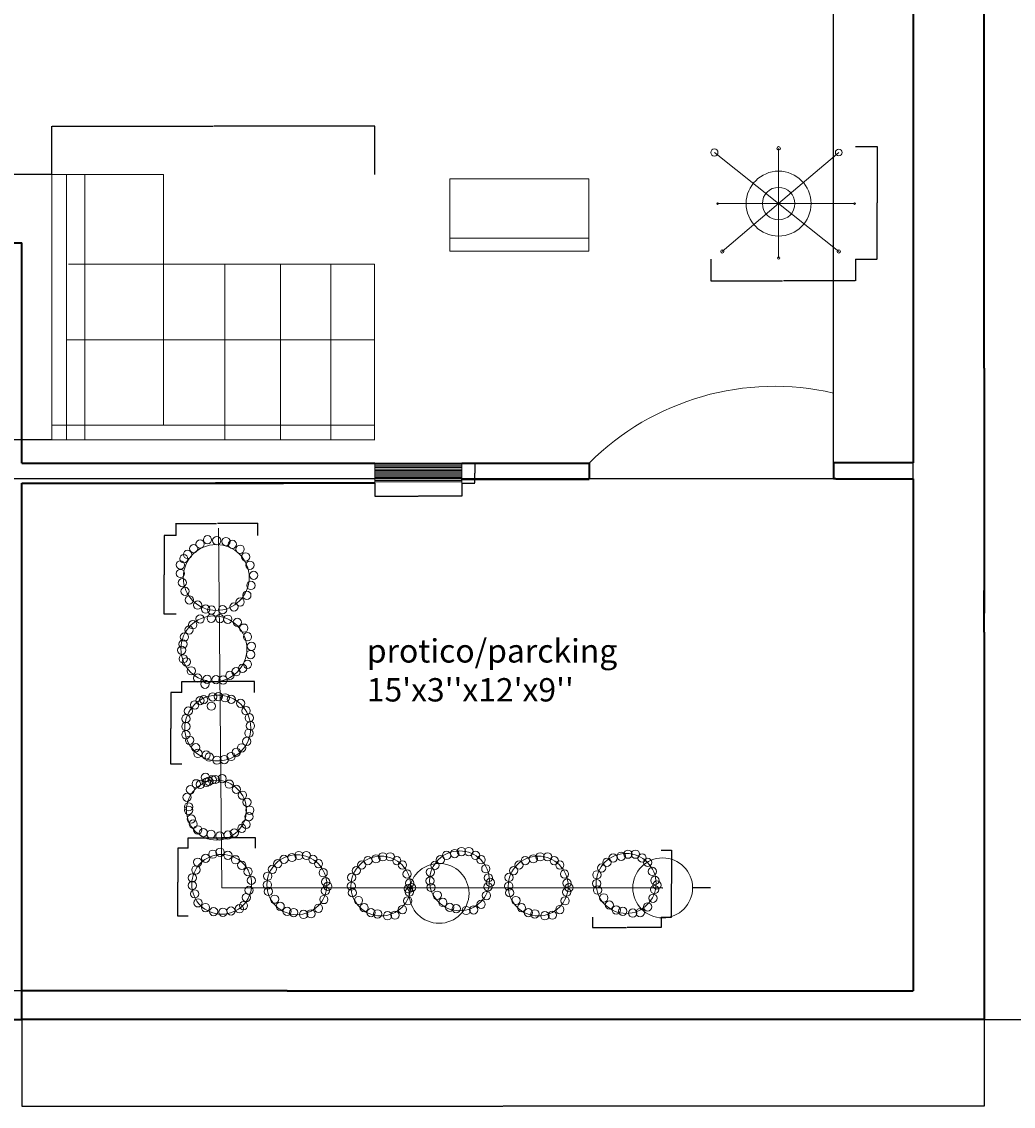
# Model space of a CAD drawing. Units: millimetres. Extents: x 1942 to 12281, y -2698 to 3078.
# Tile 2 of 6: x 4011 to 6981, y -2698 to 552. Entities that reach past the tile are written whole.
import ezdxf

# ---------------------------------------------------------------- set-up
doc = ezdxf.new("R2010")
doc.units = ezdxf.units.MM
for name, color, linetype, lineweight in [('A-ANNO-DIMS', 2, 'Continuous', 18), ('A-AREA-IDEN', 3, 'Continuous', 18), ('A-DOOR', 4, 'Continuous', 18), ('A-FURN', 8, 'Continuous', 18), ('A-GLAZ', 4, 'Continuous', 18), ('A-GLAZ-PATT', 9, 'Continuous', 13), ('A-WALL', 7, 'Continuous', 35), ('E-LITE', 6, 'Continuous', 18), ('L-PLNT', 3, 'Continuous', 13)]:
    doc.layers.add(name, color=color, linetype=linetype, lineweight=lineweight)
doc.styles.get("Standard").update_dxf_attribs({"font": 'arial.ttf'})
doc.dimstyles.get("Standard").update_dxf_attribs({"dimtxt": 0.18, "dimasz": 0.18, "dimexe": 0.18, "dimexo": 0.0625, "dimgap": 0.09, "dimtad": 0, "dimtih": 1, "dimtoh": 1, "dimdec": 4, "dimzin": 0, "dimdsep": 46, "dimtxsty": 'Standard', "dimcen": 0.09, "dimadec": 0, "dimazin": 0, "dimtfac": 1, "dimtdec": 4, "dimtofl": 0, "dimtmove": 0, "dimatfit": 3, "dimfxl": 1, "dimtolj": 1, "dimtzin": 0, "dimarcsym": 0})

# ---------------------------------------------------------------- blocks, each defined once
blk = doc.blocks.new('SOFA-SECTIONAL')
for p, q in [((0, 794.3), (0, 0)), ((0, 794.3), (334.4, 794.3)), ((43.6, 794.3), (43.6, 0)), ((98.1, 794.3), (98.1, 0)), ((334.4, 794.3), (334.4, 43.6)), ((49.7, 525.6), (966.1, 525.6)), ((517.7, 525.6), (517.9, 0)), ((684.1, 525.6), (684.3, 0)), ((834.9, 525.6), (835.1, 0)), ((966.1, 525.6), (966.3, 0)), ((43.6, 299.6), (966.2, 299.6)), ((0, 43.6), (967.4, 43.6)), ((0, 0), (967.4, 0))]:
    blk.add_line(p, q)
blk = doc.blocks.new('SEAT-LIVING')
for p, q in [((0, 38.6), (0, 0)), ((416.9, 0), (416.9, 38.6)), ((0, 0), (416.9, 0))]:
    blk.add_line(p, q)
blk.add_lwpolyline([(0, 217.2), (416.9, 217.2), (416.9, 38.6), (0, 38.6)], close=True)
blk = doc.blocks.new('CHANDELIER-8ARM')
for p, q in [((203.2, 166), (203.2, 331.7)), ((10.7, 319.2), (10.7, 319.2)), ((203.2, 166), (10.7, 319.2)), ((203.2, 166), (383.4, 319.2)), ((203.2, 166), (20.4, 166)), ((203.2, 166), (34.5, 22.7)), ((203.2, 166), (430.7, 166)), ((203.2, 166), (203.2, 3.4)), ((203.2, 166), (383.4, 22.7))]:
    blk.add_line(p, q)
for centre, radius in [((10.7, 319.2), 10.7), ((203.2, 331.7), 5.5), ((383.4, 319.2), 10.2), ((203.2, 166), 97.3), ((203.2, 166), 97.3), ((203.2, 166), 48.7), ((20.4, 166), 2.45), ((430.7, 166), 2.45), ((34.5, 22.7), 4.8), ((203.2, 3.4), 3.36), ((383.4, 22.7), 4.98)]:
    blk.add_circle(centre, radius)
blk = doc.blocks.new('DOOR-ENTRY')
blk.add_line((731.8, 0.7), (731.8, 209.8))
blk.add_arc((555.2, -555.3), 785.2, 77.0012, 134.997)
blk = doc.blocks.new('PLANT-ROUND')
for centre, radius in [((86.1, 183), 12.4), ((106.4, 189), 12.4), ((128.8, 189), 12.4), ((100.7, 101.4), 89.7), ((43.2, 164.4), 12.4), ((61.8, 177.4), 12.4), ((148.6, 177.4), 12.4), ((165.4, 164.4), 12.4), ((13.3, 127.1), 12.4), ((27.3, 147.6), 12.4), ((179.4, 137.3), 12.4), ((12.4, 101), 12.4), ((186.9, 110.3), 12.4), ((193.1, 96.5), 12.4), ((15.2, 81.4), 12.4), ((33.8, 58.1), 12.4), ((181.3, 57.1), 12.4), ((185.9, 83.2), 12.4), ((50.6, 36.6), 12.4), ((71.2, 21.7), 12.4), ((165.4, 31), 12.4), ((90.8, 18), 12.4), ((120.6, 12.4), 12.4), ((143, 14.2), 12.4)]:
    blk.add_circle(centre, radius)
blk = doc.blocks.new('PLANT-ROUND-2')
for centre, radius in [((93.4, 223.1), 12.4), ((121.1, 220.4), 12.4), ((148.7, 217.6), 12.4), ((119.6, 109.8), 98.8), ((52, 196.4), 12.4), ((71.3, 210.2), 12.4), ((168, 209.3), 12.4), ((191, 194.6), 12.4), ((22.5, 166.1), 12.4), ((33.6, 178.9), 12.4), ((207.6, 171.6), 12.4), ((12.4, 147.7), 12.4), ((12.4, 121.9), 12.4), ((220.5, 146.7), 12.4), ((17.9, 94.3), 12.4), ((223.3, 86), 12.4), ((231.6, 116.4), 12.4), ((26.2, 68.5), 12.4), ((211.3, 56.6), 12.4), ((39.1, 42.8), 12.4), ((64, 27.1), 12.4), ((172.6, 21.6), 12.4), ((191, 36.3), 12.4), ((87.9, 15.1), 12.4), ((105.4, 12.4), 12.4), ((138.6, 13.3), 12.4)]:
    blk.add_circle(centre, radius)
blk = doc.blocks.new('PLANT-ROUND-3')
for centre, radius in [((108.8, 118.6), 98.8), ((45.5, 190.7), 12.4), ((67.6, 208.2), 12.4), ((100.8, 210), 12.4), ((126.6, 209.1), 12.4), ((150.5, 207.3), 12.4), ((179.1, 198.1), 12.4), ((20.7, 153.9), 12.4), ((34.5, 175.1), 12.4), ((198.4, 180.6), 12.4), ((209.5, 154.8), 12.4), ((16.1, 132.7), 12.4), ((221.4, 126.3), 12.4), ((12.4, 114.3), 12.4), ((17, 88.6), 12.4), ((218.7, 101.4), 12.4), ((26.2, 79.4), 12.4), ((40.9, 52.7), 12.4), ((194.7, 60), 12.4), ((209.5, 72), 12.4), ((60.1, 30.8), 12.4), ((88.6, 27.1), 12.4), ((115.3, 26.2), 12.4), ((136.5, 25.3), 12.4), ((156.7, 39.1), 12.4), ((175.4, 49.9), 12.4), ((82.2, 12.4), 12.4), ((82.2, 12.4), 12.4), ((82.2, 12.4), 12.4)]:
    blk.add_circle(centre, radius)
blk = doc.blocks.new('PLANT-ROUND-4')
for centre, radius in [((108, 108.9), 98.8), ((54.7, 190.9), 12.4), ((65.8, 193.7), 12.4), ((92.5, 202), 12.4), ((110, 202.9), 12.4), ((130.3, 199.2), 12.4), ((148.7, 194.6), 12.4), ((176.3, 182.6), 12.4), ((19.8, 159.6), 12.4), ((39.1, 178), 12.4), ((88.8, 174.3), 12.4), ((88.8, 174.3), 12.4), ((88.8, 174.3), 12.4), ((88.8, 174.3), 12.4), ((192.9, 160.5), 12.4), ((12.4, 136.6), 12.4), ((202.1, 139.4), 12.4), ((12.4, 113.6), 12.4), ((12.4, 88.8), 12.4), ((201.2, 93.4), 12.4), ((205.8, 115.5), 12.4), ((23.4, 72.2), 12.4), ((194.7, 68.5), 12.4), ((41.9, 50.1), 12.4), ((48.3, 32.6), 12.4), ((73.2, 28), 12.4), ((82.4, 21.6), 12.4), ((147.8, 23.4), 12.4), ((163.4, 36.3), 12.4), ((179.1, 49.2), 12.4), ((105.4, 12.4), 12.4), ((127.5, 14.2), 12.4)]:
    blk.add_circle(centre, radius)
blk = doc.blocks.new('PLANT-ROUND-5')
for centre, radius in [((67.6, 188.1), 12.4), ((117.6, 184.4), 12.4), ((22.5, 151.3), 12.4), ((100.5, 89.8), 89.7), ((40, 168.8), 12.4), ((52, 167), 12.4), ((70.4, 173.4), 12.4), ((77.8, 176.2), 12.4), ((87.9, 180.8), 12.4), ((97.1, 181.7), 12.4), ((138.8, 167.8), 12.4), ((159.9, 152.2), 12.4), ((12.4, 128.3), 12.4), ((178.4, 134.7), 12.4), ((17, 99.8), 12.4), ((17, 89.7), 12.4), ((192.2, 113.5), 12.4), ((200.5, 89.6), 12.4), ((25, 63.2), 12.4), ((25, 63.2), 12.4), ((25, 63.2), 12.4), ((25, 63.2), 12.4), ((25, 63.2), 12.4), ((25, 63.2), 12.4), ((197.7, 70.3), 12.4), ((30.8, 48.3), 12.4), ((44.6, 30.8), 12.4), ((61.2, 22.5), 12.4), ((154.2, 21.6), 12.4), ((176.5, 35.3), 12.4), ((189.4, 47.2), 12.4), ((84.2, 17.9), 12.4), ((110.9, 12.4), 12.4), ((134.9, 15.1), 12.4)]:
    blk.add_circle(centre, radius)
blk = doc.blocks.new('PLANT-ROUND-6')
for centre, radius in [((74, 186.3), 12.4), ((95.8, 192.1), 12.4), ((119.1, 182.8), 12.4), ((100.5, 95.9), 89.7), ((28.8, 162.1), 12.4), ((52.4, 174), 12.4), ((141.9, 169.4), 12.4), ((160.8, 153), 12.4), ((23.3, 139.1), 12.4), ((179.6, 133.8), 12.4), ((12.4, 115.2), 12.4), ((12.4, 92.5), 12.4), ((189.2, 107.7), 12.4), ((19.4, 67.4), 12.4), ((174.3, 56.2), 12.4), ((182.2, 78), 12.4), ((29.6, 40.4), 12.4), ((52, 26.4), 12.4), ((153.8, 22.6), 12.4), ((165.9, 32), 12.4), ((76.3, 14.2), 12.4), ((104.3, 12.4), 12.4), ((128.6, 16.1), 12.4)]:
    blk.add_circle(centre, radius)
blk = doc.blocks.new('WIN-LIVING')
for p, q in [((0, 59.6), (0, 0)), ((0, 59.6), (260.2, 59.6)), ((260.2, 0), (260.2, 59.6))]:
    blk.add_line(p, q)
blk = doc.blocks.new('*D28')
at = {"layer": 'A-ANNO-DIMS', "color": 0, "lineweight": -2, "transparency": 16777216}
for p, q in [((4101.4, 94.2), (4101.4, 239.4)), ((4101.6, 239.3), (4583.8, 239.3)), ((5068.6, 239.3), (4586.5, 239.3)), ((5068.8, 94.2), (5068.8, 239.4))]:
    blk.add_line(p, q, dxfattribs=at)
at = {"layer": 'A-ANNO-DIMS', "color": 0, "transparency": 16777216}
for points in [[(4101.6, 239.3), (4101.6, 239.2), (4101.4, 239.3)], [(5068.6, 239.3), (5068.6, 239.2), (5068.8, 239.3)]]:
    blk.add_solid(points, dxfattribs=at)
at = {"layer": 'Defpoints', "color": 0, "transparency": 16777216}
for p in [(5068.8, 239.3), (4101.4, 94.1), (5068.8, 94.1)]:
    blk.add_point(p, dxfattribs=at)
at = {"layer": 'A-ANNO-DIMS', "color": 0, "transparency": 16777216, "insert": (4585.1, 239.3), "char_height": 0.18, "attachment_point": 5}
blk.add_mtext('\\A1;SECTIONAL 967 TYP.', dxfattribs=at)
blk = doc.blocks.new('*D29')
at = {"layer": 'A-ANNO-DIMS', "color": 0, "lineweight": -2, "transparency": 16777216}
for p, q in [((4101.3, 94.1), (3956.1, 94.1)), ((3956.3, 94), (3956.3, -302.8)), ((3956.3, -700), (3956.3, -303.2)), ((4101.3, -700.2), (3956.1, -700.2))]:
    blk.add_line(p, q, dxfattribs=at)
at = {"layer": 'A-ANNO-DIMS', "color": 0, "transparency": 16777216}
for points in [[(3956.3, 94), (3956.3, 94), (3956.3, 94.1)], [(3956.3, -700), (3956.3, -700), (3956.3, -700.2)]]:
    blk.add_solid(points, dxfattribs=at)
at = {"layer": 'Defpoints', "color": 0, "transparency": 16777216}
for p in [(3956.3, 94.1), (4101.4, 94.1), (4101.4, -700.2)]:
    blk.add_point(p, dxfattribs=at)
at = {"layer": 'A-ANNO-DIMS', "color": 0, "transparency": 16777216, "insert": (3956.3, -303), "char_height": 0.18, "attachment_point": 5}
blk.add_mtext('\\A1;794 TYP.', dxfattribs=at)
blk = doc.blocks.new('*D32')
at = {"layer": 'A-ANNO-DIMS', "color": 0, "lineweight": -2, "transparency": 16777216}
for p, q in [((6075.1, -158.9), (6075.1, -224)), ((6508.2, -158.9), (6508.2, -224)), ((6075.2, -223.8), (6290.2, -223.8)), ((6508, -223.8), (6293.1, -223.8))]:
    blk.add_line(p, q, dxfattribs=at)
at = {"layer": 'A-ANNO-DIMS', "color": 0, "transparency": 16777216}
for points in [[(6075.2, -223.8), (6075.2, -223.9), (6075.1, -223.8)], [(6508, -223.8), (6508, -223.9), (6508.2, -223.8)]]:
    blk.add_solid(points, dxfattribs=at)
at = {"layer": 'Defpoints', "color": 0, "transparency": 16777216}
for p in [(6075.1, -158.9), (6508.2, -158.9), (6508.2, -223.8)]:
    blk.add_point(p, dxfattribs=at)
at = {"layer": 'A-ANNO-DIMS', "color": 0, "transparency": 16777216, "insert": (6291.6, -223.8), "char_height": 0.18, "attachment_point": 5}
blk.add_mtext('\\A1;CHANDELIER 433 TYP.', dxfattribs=at)
blk = doc.blocks.new('*D33')
at = {"layer": 'A-ANNO-DIMS', "color": 0, "lineweight": -2, "transparency": 16777216}
for p, q in [((6508.3, 178.4), (6573.3, 178.4)), ((6573.2, 178.2), (6573.2, 9.9)), ((6573.2, -158.7), (6573.2, 9.6)), ((6508.3, -158.9), (6573.3, -158.9))]:
    blk.add_line(p, q, dxfattribs=at)
at = {"layer": 'A-ANNO-DIMS', "color": 0, "transparency": 16777216}
for points in [[(6573.1, 178.2), (6573.2, 178.2), (6573.2, 178.4)], [(6573.1, -158.7), (6573.2, -158.7), (6573.2, -158.9)]]:
    blk.add_solid(points, dxfattribs=at)
at = {"layer": 'Defpoints', "color": 0, "transparency": 16777216}
for p in [(6508.2, 178.4), (6573.2, 178.4), (6508.2, -158.9)]:
    blk.add_point(p, dxfattribs=at)
at = {"layer": 'A-ANNO-DIMS', "color": 0, "transparency": 16777216, "insert": (6573.2, 9.8), "char_height": 0.18, "attachment_point": 5}
blk.add_mtext('\\A1;337 TYP.', dxfattribs=at)
blk = doc.blocks.new('*D48')
at = {"layer": 'A-ANNO-DIMS', "color": 0, "lineweight": -2, "transparency": 16777216}
for p, q in [((5720.6, -2131.3), (5720.6, -2162.2)), ((5926.1, -2131.3), (5926.1, -2162.2)), ((5720.8, -2162), (5822.2, -2162)), ((5925.9, -2162), (5824.5, -2162))]:
    blk.add_line(p, q, dxfattribs=at)
at = {"layer": 'A-ANNO-DIMS', "color": 0, "transparency": 16777216}
for points in [[(5720.8, -2162), (5720.8, -2162.1), (5720.6, -2162)], [(5925.9, -2162), (5925.9, -2162.1), (5926.1, -2162)]]:
    blk.add_solid(points, dxfattribs=at)
at = {"layer": 'Defpoints', "color": 0, "transparency": 16777216}
for p in [(5720.6, -2131.2), (5926.1, -2131.2), (5926.1, -2162)]:
    blk.add_point(p, dxfattribs=at)
at = {"layer": 'A-ANNO-DIMS', "color": 0, "transparency": 16777216, "insert": (5823.3, -2162), "char_height": 0.18, "attachment_point": 5}
blk.add_mtext('\\A1;PLANT A 205 TYP.', dxfattribs=at)
blk = doc.blocks.new('*D49')
at = {"layer": 'A-ANNO-DIMS', "color": 0, "lineweight": -2, "transparency": 16777216}
for p, q in [((5926.1, -1929.9), (5957.1, -1929.9)), ((5956.9, -1930.1), (5956.9, -2030.4)), ((5956.9, -2131), (5956.9, -2030.7)), ((5926.1, -2131.2), (5957.1, -2131.2))]:
    blk.add_line(p, q, dxfattribs=at)
at = {"layer": 'A-ANNO-DIMS', "color": 0, "transparency": 16777216}
for points in [[(5956.9, -1930.1), (5956.9, -1930.1), (5956.9, -1929.9)], [(5956.9, -2131), (5956.9, -2131), (5956.9, -2131.2)]]:
    blk.add_solid(points, dxfattribs=at)
at = {"layer": 'Defpoints', "color": 0, "transparency": 16777216}
for p in [(5926.1, -1929.9), (5956.9, -1929.9), (5926.1, -2131.2)]:
    blk.add_point(p, dxfattribs=at)
at = {"layer": 'A-ANNO-DIMS', "color": 0, "transparency": 16777216, "insert": (5956.9, -2030.5), "char_height": 0.18, "attachment_point": 5}
blk.add_mtext('\\A1;201 TYP.', dxfattribs=at)
blk = doc.blocks.new('*D50')
at = {"layer": 'A-ANNO-DIMS', "color": 0, "lineweight": -2, "transparency": 16777216}
for p, q in [((4473.9, -987.4), (4473.9, -950.7)), ((4474.1, -950.9), (4594.7, -950.9)), ((4717.7, -950.9), (4597, -950.9)), ((4717.9, -987.4), (4717.9, -950.7))]:
    blk.add_line(p, q, dxfattribs=at)
at = {"layer": 'A-ANNO-DIMS', "color": 0, "transparency": 16777216}
for points in [[(4474.1, -950.9), (4474.1, -950.9), (4473.9, -950.9)], [(4717.7, -950.9), (4717.7, -950.9), (4717.9, -950.9)]]:
    blk.add_solid(points, dxfattribs=at)
at = {"layer": 'Defpoints', "color": 0, "transparency": 16777216}
for p in [(4717.9, -950.9), (4473.9, -987.5), (4717.9, -987.5)]:
    blk.add_point(p, dxfattribs=at)
at = {"layer": 'A-ANNO-DIMS', "color": 0, "transparency": 16777216, "insert": (4595.9, -950.9), "char_height": 0.18, "attachment_point": 5}
blk.add_mtext('\\A1;PLANT B 244 TYP.', dxfattribs=at)
blk = doc.blocks.new('*D51')
at = {"layer": 'A-ANNO-DIMS', "color": 0, "lineweight": -2, "transparency": 16777216}
for p, q in [((4473.9, -987.5), (4437.1, -987.5)), ((4437.3, -987.7), (4437.3, -1105.1)), ((4437.3, -1222.8), (4437.3, -1105.4)), ((4473.9, -1223), (4437.1, -1223))]:
    blk.add_line(p, q, dxfattribs=at)
at = {"layer": 'A-ANNO-DIMS', "color": 0, "transparency": 16777216}
for points in [[(4437.3, -987.7), (4437.4, -987.7), (4437.3, -987.5)], [(4437.3, -1222.8), (4437.4, -1222.8), (4437.3, -1223)]]:
    blk.add_solid(points, dxfattribs=at)
at = {"layer": 'Defpoints', "color": 0, "transparency": 16777216}
for p in [(4437.3, -987.5), (4473.9, -987.5), (4473.9, -1223)]:
    blk.add_point(p, dxfattribs=at)
at = {"layer": 'A-ANNO-DIMS', "color": 0, "transparency": 16777216, "insert": (4437.3, -1105.2), "char_height": 0.18, "attachment_point": 5}
blk.add_mtext('\\A1;236 TYP.', dxfattribs=at)
blk = doc.blocks.new('*D54')
at = {"layer": 'A-ANNO-DIMS', "color": 0, "lineweight": -2, "transparency": 16777216}
for p, q in [((4490.2, -1457.6), (4490.2, -1424.8)), ((4490.3, -1424.9), (4598.1, -1424.9)), ((4708.1, -1424.9), (4600.4, -1424.9)), ((4708.3, -1457.6), (4708.3, -1424.8))]:
    blk.add_line(p, q, dxfattribs=at)
at = {"layer": 'A-ANNO-DIMS', "color": 0, "transparency": 16777216}
for points in [[(4490.3, -1424.9), (4490.3, -1425), (4490.2, -1424.9)], [(4708.1, -1424.9), (4708.1, -1425), (4708.3, -1424.9)]]:
    blk.add_solid(points, dxfattribs=at)
at = {"layer": 'Defpoints', "color": 0, "transparency": 16777216}
for p in [(4708.3, -1424.9), (4490.2, -1457.7), (4708.3, -1457.7)]:
    blk.add_point(p, dxfattribs=at)
at = {"layer": 'A-ANNO-DIMS', "color": 0, "transparency": 16777216, "insert": (4599.2, -1424.9), "char_height": 0.18, "attachment_point": 5}
blk.add_mtext('\\A1;PLANT D 218 TYP.', dxfattribs=at)
blk = doc.blocks.new('*D55')
at = {"layer": 'A-ANNO-DIMS', "color": 0, "lineweight": -2, "transparency": 16777216}
for p, q in [((4490.1, -1457.7), (4457.3, -1457.7)), ((4457.4, -1457.9), (4457.4, -1565.1)), ((4457.4, -1672.8), (4457.4, -1565.5)), ((4490.1, -1672.9), (4457.3, -1672.9))]:
    blk.add_line(p, q, dxfattribs=at)
at = {"layer": 'A-ANNO-DIMS', "color": 0, "transparency": 16777216}
for points in [[(4457.4, -1457.9), (4457.5, -1457.9), (4457.4, -1457.7)], [(4457.4, -1672.8), (4457.5, -1672.8), (4457.4, -1672.9)]]:
    blk.add_solid(points, dxfattribs=at)
at = {"layer": 'Defpoints', "color": 0, "transparency": 16777216}
for p in [(4457.4, -1457.7), (4490.2, -1457.7), (4490.2, -1672.9)]:
    blk.add_point(p, dxfattribs=at)
at = {"layer": 'A-ANNO-DIMS', "color": 0, "transparency": 16777216, "insert": (4457.4, -1565.3), "char_height": 0.18, "attachment_point": 5}
blk.add_mtext('\\A1;215 TYP.', dxfattribs=at)
blk = doc.blocks.new('*D58')
at = {"layer": 'A-ANNO-DIMS', "color": 0, "lineweight": -2, "transparency": 16777216}
for p, q in [((4509.2, -1923.9), (4478.4, -1923.9)), ((4478.6, -1924.1), (4478.6, -2026)), ((4478.6, -2128.3), (4478.6, -2026.4)), ((4509.2, -2128.4), (4478.4, -2128.4))]:
    blk.add_line(p, q, dxfattribs=at)
at = {"layer": 'A-ANNO-DIMS', "color": 0, "transparency": 16777216}
for points in [[(4478.6, -1924.1), (4478.6, -1924.1), (4478.6, -1923.9)], [(4478.6, -2128.3), (4478.6, -2128.3), (4478.6, -2128.4)]]:
    blk.add_solid(points, dxfattribs=at)
at = {"layer": 'Defpoints', "color": 0, "transparency": 16777216}
for p in [(4478.6, -1923.9), (4509.3, -1923.9), (4509.3, -2128.4)]:
    blk.add_point(p, dxfattribs=at)
at = {"layer": 'A-ANNO-DIMS', "color": 0, "transparency": 16777216, "insert": (4478.6, -2026.2), "char_height": 0.18, "attachment_point": 5}
blk.add_mtext('\\A1;PLANT F 204 TYP.', dxfattribs=at)
blk = doc.blocks.new('*D59')
at = {"layer": 'A-ANNO-DIMS', "color": 0, "lineweight": -2, "transparency": 16777216}
for p, q in [((4509.3, -1923.9), (4509.3, -1893.1)), ((4509.4, -1893.3), (4609.5, -1893.3)), ((4710.7, -1893.3), (4610.7, -1893.3)), ((4710.8, -1923.9), (4710.8, -1893.1))]:
    blk.add_line(p, q, dxfattribs=at)
at = {"layer": 'A-ANNO-DIMS', "color": 0, "transparency": 16777216}
for points in [[(4509.4, -1893.2), (4509.4, -1893.3), (4509.3, -1893.3)], [(4710.7, -1893.2), (4710.7, -1893.3), (4710.8, -1893.3)]]:
    blk.add_solid(points, dxfattribs=at)
at = {"layer": 'Defpoints', "color": 0, "transparency": 16777216}
for p in [(4710.8, -1893.3), (4509.3, -1923.9), (4710.8, -1923.9)]:
    blk.add_point(p, dxfattribs=at)
at = {"layer": 'A-ANNO-DIMS', "color": 0, "transparency": 16777216, "insert": (4610.1, -1893.3), "char_height": 0.18, "attachment_point": 5}
blk.add_mtext('\\A1;202 TYP.', dxfattribs=at)
blk = doc.blocks.new('*D68')
at = {"layer": 'A-ANNO-DIMS', "color": 0, "lineweight": -2, "transparency": 16777216}
for p, q in [((5068.8, -830.1), (5068.8, -869.2)), ((5329.1, -830.1), (5329.1, -869.2)), ((5069, -869.1), (5198.1, -869.1)), ((5328.9, -869.1), (5199.8, -869.1))]:
    blk.add_line(p, q, dxfattribs=at)
at = {"layer": 'A-ANNO-DIMS', "color": 0, "transparency": 16777216}
for points in [[(5069, -869), (5069, -869.1), (5068.8, -869.1)], [(5328.9, -869), (5328.9, -869.1), (5329.1, -869.1)]]:
    blk.add_solid(points, dxfattribs=at)
at = {"layer": 'Defpoints', "color": 0, "transparency": 16777216}
for p in [(5068.8, -830), (5329.1, -830), (5329.1, -869.1)]:
    blk.add_point(p, dxfattribs=at)
at = {"layer": 'A-ANNO-DIMS', "color": 0, "transparency": 16777216, "insert": (5199, -869.1), "char_height": 0.18, "attachment_point": 5}
blk.add_mtext('\\A1;W5 260 TYP.', dxfattribs=at)
blk = doc.blocks.new('*D69')
at = {"layer": 'A-ANNO-DIMS', "color": 0, "lineweight": -2, "transparency": 16777216}
for p, q in [((5329.1, -770.4), (5368.3, -770.4)), ((5368.1, -770.6), (5368.1, -800)), ((5368.1, -829.8), (5368.1, -800.4)), ((5329.1, -830), (5368.3, -830))]:
    blk.add_line(p, q, dxfattribs=at)
at = {"layer": 'A-ANNO-DIMS', "color": 0, "transparency": 16777216}
for points in [[(5368.1, -770.6), (5368.1, -770.6), (5368.1, -770.4)], [(5368.1, -829.8), (5368.1, -829.8), (5368.1, -830)]]:
    blk.add_solid(points, dxfattribs=at)
at = {"layer": 'Defpoints', "color": 0, "transparency": 16777216}
for p in [(5329.1, -770.4), (5368.1, -770.4), (5329.1, -830)]:
    blk.add_point(p, dxfattribs=at)
at = {"layer": 'A-ANNO-DIMS', "color": 0, "transparency": 16777216, "insert": (5368.1, -800.2), "char_height": 0.18, "attachment_point": 5}
blk.add_mtext('\\A1;60 TYP.', dxfattribs=at)
blk = doc.blocks.new('*D71')
at = {"layer": 'A-ANNO-DIMS', "color": 0, "lineweight": -2, "transparency": 16777216}
for p, q in [((6894.2, 2765.9), (7154.5, 2765.9)), ((7154.3, 2765.7), (7154.3, 164.5)), ((7154.3, -2437.1), (7154.3, 164.1)), ((6894.2, -2437.2), (7154.5, -2437.2))]:
    blk.add_line(p, q, dxfattribs=at)
at = {"layer": 'A-ANNO-DIMS', "color": 0, "transparency": 16777216}
for points in [[(7154.3, 2765.7), (7154.4, 2765.7), (7154.3, 2765.9)], [(7154.3, -2437.1), (7154.4, -2437.1), (7154.3, -2437.2)]]:
    blk.add_solid(points, dxfattribs=at)
at = {"layer": 'Defpoints', "color": 0, "transparency": 16777216}
for p in [(6894.1, 2765.9), (7154.3, 2765.9), (6894.1, -2437.2)]:
    blk.add_point(p, dxfattribs=at)
at = {"layer": 'A-ANNO-DIMS', "color": 0, "transparency": 16777216, "insert": (7154.3, 164.3), "char_height": 0.18, "attachment_point": 5}
blk.add_mtext('\\A1;5203', dxfattribs=at)
blk = doc.blocks.new('*D73')
at = {"layer": 'A-ANNO-DIMS', "color": 0, "lineweight": -2, "transparency": 16777216}
for p, q in [((4010.7, -2437.3), (4010.7, -2697.7)), ((6894.1, -2437.3), (6894.1, -2697.7)), ((4010.9, -2697.5), (5451.9, -2697.5)), ((6893.9, -2697.5), (5452.9, -2697.5))]:
    blk.add_line(p, q, dxfattribs=at)
at = {"layer": 'A-ANNO-DIMS', "color": 0, "transparency": 16777216}
for points in [[(4010.9, -2697.5), (4010.9, -2697.5), (4010.7, -2697.5)], [(6893.9, -2697.5), (6893.9, -2697.5), (6894.1, -2697.5)]]:
    blk.add_solid(points, dxfattribs=at)
at = {"layer": 'Defpoints', "color": 0, "transparency": 16777216}
for p in [(4010.7, -2437.2), (6894.1, -2437.2), (6894.1, -2697.5)]:
    blk.add_point(p, dxfattribs=at)
at = {"layer": 'A-ANNO-DIMS', "color": 0, "transparency": 16777216, "insert": (5452.4, -2697.5), "char_height": 0.18, "attachment_point": 5}
blk.add_mtext('\\A1;2883.4', dxfattribs=at)
blk = doc.blocks.new('*D81')
at = {"layer": 'A-ANNO-DIMS', "color": 0, "lineweight": -2, "transparency": 16777216}
for p, q in [((6681.4, -817), (1942, -817)), ((1942.2, -817.2), (1942.2, -1584.1)), ((1942.2, -2351.4), (1942.2, -1584.5)), ((6681.4, -2351.6), (1942, -2351.6))]:
    blk.add_line(p, q, dxfattribs=at)
at = {"layer": 'A-ANNO-DIMS', "color": 0, "transparency": 16777216}
for points in [[(1942.2, -817.2), (1942.2, -817.2), (1942.2, -817)], [(1942.2, -2351.4), (1942.2, -2351.4), (1942.2, -2351.6)]]:
    blk.add_solid(points, dxfattribs=at)
at = {"layer": 'Defpoints', "color": 0, "transparency": 16777216}
for p in [(1942.2, -817), (6681.5, -817), (6681.5, -2351.6)]:
    blk.add_point(p, dxfattribs=at)
at = {"layer": 'A-ANNO-DIMS', "color": 0, "transparency": 16777216, "insert": (1942.2, -1584.3), "char_height": 0.18, "attachment_point": 5}
blk.add_mtext('\\A1;1534.5', dxfattribs=at)
blk = doc.blocks.new('*D82')
at = {"layer": 'A-ANNO-DIMS', "color": 0, "lineweight": -2, "transparency": 16777216}
for p, q in [((6442.7, -769.4), (6442.7, 3026.3)), ((6442.9, 3026.1), (6561.6, 3026.1)), ((6681.3, 3026.1), (6562.6, 3026.1)), ((6681.5, -769.5), (6681.5, 3026.3))]:
    blk.add_line(p, q, dxfattribs=at)
at = {"layer": 'A-ANNO-DIMS', "color": 0, "transparency": 16777216}
for points in [[(6442.9, 3026.2), (6442.9, 3026.1), (6442.7, 3026.1)], [(6681.3, 3026.2), (6681.3, 3026.1), (6681.5, 3026.1)]]:
    blk.add_solid(points, dxfattribs=at)
at = {"layer": 'Defpoints', "color": 0, "transparency": 16777216}
for p in [(6681.5, 3026.1), (6442.7, -769.5), (6681.5, -769.5)]:
    blk.add_point(p, dxfattribs=at)
at = {"layer": 'A-ANNO-DIMS', "color": 0, "transparency": 16777216, "insert": (6562.1, 3026.1), "char_height": 0.18, "attachment_point": 5}
blk.add_mtext('\\A1;238.74', dxfattribs=at)
blk = doc.blocks.new('*D90')
at = {"layer": 'A-ANNO-DIMS', "color": 0, "lineweight": -2, "transparency": 16777216}
for p, q in [((6681.5, -2351.5), (6681.5, 3026.3)), ((6681.6, 3026.1), (6787.3, 3026.1)), ((6893.9, 3026.1), (6788.2, 3026.1)), ((6894.1, -2437.2), (6894.1, 3026.3))]:
    blk.add_line(p, q, dxfattribs=at)
at = {"layer": 'A-ANNO-DIMS', "color": 0, "transparency": 16777216}
for points in [[(6681.6, 3026.2), (6681.6, 3026.1), (6681.5, 3026.1)], [(6893.9, 3026.2), (6893.9, 3026.1), (6894.1, 3026.1)]]:
    blk.add_solid(points, dxfattribs=at)
at = {"layer": 'Defpoints', "color": 0, "transparency": 16777216}
for p in [(6894.1, 3026.1), (6681.5, -2351.6), (6894.1, -2437.2)]:
    blk.add_point(p, dxfattribs=at)
at = {"layer": 'A-ANNO-DIMS', "color": 0, "transparency": 16777216, "insert": (6787.8, 3026.1), "char_height": 0.18, "attachment_point": 5}
blk.add_mtext('\\A1;212.64', dxfattribs=at)
blk = doc.blocks.new('*D122')
at = {"layer": 'A-ANNO-DIMS', "color": 0, "lineweight": -2, "transparency": 16777216}
for p, q in [((5930.8, -2043.2), (5931, -2043.2)), ((5930.9, -2043.3), (5930.9, -2043.1)), ((6074.4, -2043.2), (6020.7, -2043.2))]:
    blk.add_line(p, q, dxfattribs=at)
at = {"layer": 'A-ANNO-DIMS', "color": 0, "transparency": 16777216}
blk.add_solid([(6020.7, -2043.2), (6020.7, -2043.2), (6020.5, -2043.2)], dxfattribs=at)
at = {"layer": 'Defpoints', "color": 0, "transparency": 16777216}
for p in [(5841.2, -2043.2), (6020.5, -2043.2)]:
    blk.add_point(p, dxfattribs=at)
at = {"layer": 'A-ANNO-DIMS', "color": 0, "transparency": 16777216, "insert": (6075.2, -2043.2), "char_height": 0.18, "attachment_point": 5}
blk.add_mtext('\\A1;18X ∅179.38', dxfattribs=at)

msp = doc.modelspace()

# ---------------------------------------------------------------- hatches: boundary and pattern name
at = {"layer": 'A-GLAZ-PATT'}
h = msp.add_hatch(dxfattribs=at)
h.set_pattern_fill('ANSI31', color=256, scale=1.34183, angle=135, style=0)
h.paths.add_polyline_path([(5068.829, -830.024), (5329.073, -830.024), (5329.073, -770.379), (5068.829, -770.379)])

# ---------------------------------------------------------------- linework, layer by layer
at = {"layer": 'A-WALL'}
for p, q in [((6894.096, -486.223), (6894.096, 2765.873)), ((6681.459, 2491.56), (6681.459, -486.223)), ((3945.31, -110.599), (4010.712, -110.599)), ((4010.712, -770.379), (4010.712, -110.599)), ((6681.459, -486.223), (6681.459, -769.472)), ((6894.096, -486.223), (6894.096, -1220.435)), ((4010.712, -770.379), (4795.23, -770.379)), ((4795.23, -770.379), (4795.23, -770.379)), ((4795.23, -770.379), (5068.829, -770.379)), ((5329.073, -770.379), (5710.887, -770.14)), ((5710.887, -770.14), (5710.887, -818.204)), ((6681.459, -769.472), (6442.72, -769.472)), ((6442.72, -769.472), (6442.72, -817.04)), ((6681.459, -769.472), (6681.459, -769.531)), ((6681.459, -769.472), (6681.459, -769.531)), ((4010.712, -1820.671), (4010.712, -830.024)), ((4010.712, -830.024), (4795.23, -830.024)), ((4591.655, -829.715), (4851.9, -829.715)), ((4591.655, -829.715), (4851.9, -829.715)), ((4591.655, -829.715), (4851.9, -829.715)), ((4591.655, -829.715), (4851.9, -829.715)), ((4591.655, -829.715), (4851.9, -829.715)), ((4591.655, -829.715), (4851.9, -829.715)), ((4591.655, -829.715), (4851.9, -829.715)), ((4591.655, -829.715), (4851.9, -829.715)), ((5068.829, -830.024), (4795.23, -830.024)), ((5327.06, -818.665), (5710.887, -818.204)), ((6449.441, -817.04), (6442.72, -817.04)), ((6449.441, -817.04), (6681.459, -817.04)), ((6681.459, -817.04), (6681.459, -1062.931)), ((6681.459, -1062.931), (6681.459, -1277.224)), ((6894.096, -1277.224), (6894.096, -1151.652)), ((6681.459, -1277.224), (6681.459, -2351.554)), ((6894.096, -1277.224), (6894.096, -2437.233)), ((4010.712, -2437.233), (4010.712, -1820.671)), ((4010.712, -1820.671), (4010.712, -1820.671)), ((4805.662, -2351.554), (4010.712, -2351.554)), ((4805.662, -2351.554), (6681.459, -2351.554)), ((3380.631, -2437.233), (4010.712, -2437.233)), ((4805.662, -2437.233), (4010.712, -2437.233)), ((6894.096, -2437.233), (4805.662, -2437.233))]:
    msp.add_line(p, q, dxfattribs=at)
at = {"layer": 'L-PLNT'}
for p, q in [((4600.545, -965.181), (4609.947, -2043.199)), ((4609.947, -2043.199), (5930.86, -2043.199)), ((5930.86, -2043.199), (5930.86, -2043.199))]:
    msp.add_line(p, q, dxfattribs=at)
for centre, radius in [((5261.002, -2059.639), 89.689), ((5930.86, -2043.199), 89.689), ((5168.968, -2045.803), 12.385)]:
    msp.add_circle(centre, radius, dxfattribs=at)

# ---------------------------------------------------------------- block references
at = {"layer": 'A-DOOR'}
msp.add_blockref('DOOR-ENTRY', (5710.887, -770.14), dxfattribs=at)
at = {"layer": 'A-FURN'}
for name, p in [('SOFA-SECTIONAL', (4101.403, -700.178)), ('SEAT-LIVING', (5293.245, -135.364))]:
    msp.add_blockref(name, p, dxfattribs=at)
at = {"layer": 'A-GLAZ'}
msp.add_blockref('WIN-LIVING', (5068.829, -830.024), dxfattribs=at)
at = {"layer": 'E-LITE'}
msp.add_blockref('CHANDELIER-8ARM', (6075.069, -158.866), dxfattribs=at)
at = {"layer": 'L-PLNT'}
for name, p in [('PLANT-ROUND-2', (4473.922, -1222.986)), ('PLANT-ROUND-3', (4477.606, -1445.473)), ('PLANT-ROUND-4', (4490.157, -1672.93)), ('PLANT-ROUND-5', (4493.629, -1900.123)), ('PLANT-ROUND-6', (4509.27, -2128.44)), ('PLANT-ROUND', (4734.475, -2135.144)), ('PLANT-ROUND', (4985.913, -2139.07)), ('PLANT-ROUND', (5221.637, -2123.367)), ('PLANT-ROUND', (5457.36, -2139.07)), ('PLANT-ROUND', (5720.585, -2131.218))]:
    msp.add_blockref(name, p, dxfattribs=at)

# ---------------------------------------------------------------- texts
at = {"layer": 'A-AREA-IDEN', "insert": (5044.679, -1297.974), "char_height": 70, "attachment_point": 1}
msp.add_mtext("protico/parcking\\P15'x3''x12'x9''", dxfattribs=at)

# ---------------------------------------------------------------- dimensions: what is measured, and where the dimension line sits
at = {"layer": 'A-ANNO-DIMS'}
for base, p1, p2, override, picture, middle in [((6681.459, 3026.123), (6442.72, -769.472), (6681.459, -769.531), {"dimdec": 2, "dimlfac": 1, "dimrnd": 0, "dimzin": 0, "dimdsep": 46, "dimlunit": 2}, '*D82', (6562.09, 3026.123)), ((6894.096, 3026.123), (6681.459, -2351.554), (6894.096, -2437.233), {"dimdec": 2, "dimlfac": 1, "dimrnd": 0, "dimzin": 0, "dimdsep": 46, "dimlunit": 2}, '*D90', (6787.777, 3026.123)), ((6894.096, -2697.483), (4010.712, -2437.233), (6894.096, -2437.233), {"dimdec": 1, "dimlfac": 1, "dimrnd": 0, "dimzin": 0, "dimdsep": 46, "dimlunit": 2}, '*D73', (5452.404, -2697.483))]:
    dim = msp.add_linear_dim(base=base, p1=p1, p2=p2, dimstyle='Standard', override=override, dxfattribs=at)
    dim.commit()
    dim.dimension.update_dxf_attribs({"geometry": picture, "text_midpoint": middle})
for base, p1, p2, override, picture, middle in [((7154.346, 2765.873), (6894.096, -2437.233), (6894.096, 2765.873), {"dimdec": 0, "dimlfac": 1, "dimrnd": 0, "dimzin": 0, "dimdsep": 46, "dimlunit": 2}, '*D71', (7154.346, 164.32)), ((1942.2, -817.04), (6681.459, -2351.554), (6681.459, -817.04), {"dimdec": 1, "dimlfac": 1, "dimrnd": 0, "dimzin": 0, "dimdsep": 46, "dimlunit": 2}, '*D81', (1942.2, -1584.297))]:
    dim = msp.add_linear_dim(base=base, p1=p1, p2=p2, angle=90, dimstyle='Standard', override=override, dxfattribs=at)
    dim.commit()
    dim.dimension.update_dxf_attribs({"geometry": picture, "text_midpoint": middle})
for base, p1, p2, text, picture, middle in [((5068.829, 239.263), (4101.403, 94.15), (5068.829, 94.15), 'SECTIONAL <> TYP.', '*D28', (4585.116, 239.263)), ((6508.195, -223.835), (6075.069, -158.866), (6508.195, -158.866), 'CHANDELIER <> TYP.', '*D32', (6291.632, -223.835)), ((5329.073, -869.06), (5068.829, -830.024), (5329.073, -830.024), 'W5 <> TYP.', '*D68', (5198.951, -869.06)), ((4717.871, -950.891), (4473.922, -987.483), (4717.871, -987.483), 'PLANT B <> TYP.', '*D50', (4595.897, -950.891)), ((4708.32, -1424.948), (4490.157, -1457.672), (4708.32, -1457.672), 'PLANT D <> TYP.', '*D54', (4599.238, -1424.948)), ((4710.832, -1893.266), (4509.27, -1923.941), (4710.832, -1923.941), '<> TYP.', '*D59', (4610.051, -1893.266)), ((5926.073, -2162.041), (5720.585, -2131.218), (5926.073, -2131.218), 'PLANT A <> TYP.', '*D48', (5823.329, -2162.041))]:
    dim = msp.add_linear_dim(base=base, p1=p1, p2=p2, text=text, dimstyle='Standard', override={"dimdec": 0, "dimlfac": 1, "dimrnd": 0, "dimzin": 0, "dimdsep": 46, "dimlunit": 2}, dxfattribs=at)
    dim.commit()
    dim.dimension.update_dxf_attribs({"geometry": picture, "text_midpoint": middle})
for base, p1, p2, text, picture, middle in [((6573.163, 178.387), (6508.195, -158.866), (6508.195, 178.387), '<> TYP.', '*D33', (6573.163, 9.761)), ((3956.289, 94.15), (4101.403, -700.178), (4101.403, 94.15), '<> TYP.', '*D29', (3956.289, -303.014)), ((5368.11, -770.379), (5329.073, -830.024), (5329.073, -770.379), '<> TYP.', '*D69', (5368.11, -800.202)), ((4437.33, -987.483), (4473.922, -1222.986), (4473.922, -987.483), '<> TYP.', '*D51', (4437.33, -1105.235)), ((4457.432, -1457.672), (4490.157, -1672.93), (4490.157, -1457.672), '<> TYP.', '*D55', (4457.432, -1565.301)), ((4478.595, -1923.941), (4509.27, -2128.44), (4509.27, -1923.941), 'PLANT F <> TYP.', '*D58', (4478.595, -2026.19)), ((5956.896, -1929.881), (5926.073, -2131.218), (5926.073, -1929.881), '<> TYP.', '*D49', (5956.896, -2030.55))]:
    dim = msp.add_linear_dim(base=base, p1=p1, p2=p2, angle=90, text=text, dimstyle='Standard', override={"dimdec": 0, "dimlfac": 1, "dimrnd": 0, "dimzin": 0, "dimdsep": 46, "dimlunit": 2}, dxfattribs=at)
    dim.commit()
    dim.dimension.update_dxf_attribs({"geometry": picture, "text_midpoint": middle})
dim = msp.add_diameter_dim_2p(p1=(5841.171, -2043.198), p2=(6020.55, -2043.2), text='18X <>', dimstyle='Standard', override={"dimdec": 2, "dimlfac": 1, "dimrnd": 0, "dimzin": 0, "dimdsep": 46, "dimlunit": 2}, dxfattribs=at)
dim.commit()
dim.dimension.update_dxf_attribs({"geometry": '*D122', "text_midpoint": (6074.363, -2043.201), "dimtype": 163})

doc.saveas('drawing.dxf')
